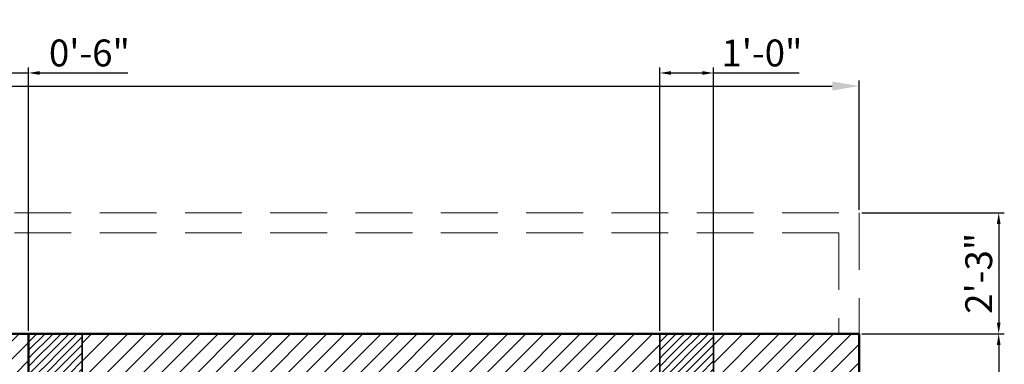
# Model space of a CAD drawing. Units: millimetres. Extents: x 225995 to 227247, y 225507 to 226008.
# Tile 10 of 23: x 226378 to 226598, y 225927 to 226004. Entities that reach past the tile are written whole.
import ezdxf

# ---------------------------------------------------------------- set-up
doc = ezdxf.new("R2010")
doc.units = ezdxf.units.MM
doc.linetypes.add('DASHED', pattern=[19.05, 12.7, -6.35])
for name, color, linetype, lineweight in [('A-ANNO-DIMS', 2, 'Continuous', 18), ('A-COLS', 40, 'Continuous', 35), ('A-WALL', 7, 'Continuous', 50), ('A-WALL-OVHD', 1, 'DASHED', 18), ('A-WALL-PATT', 8, 'Continuous', 13)]:
    doc.layers.add(name, color=color, linetype=linetype, lineweight=lineweight)
doc.styles.get("Standard").update_dxf_attribs({"font": 'arial.ttf'})
doc.dimstyles.new('ISO-25', dxfattribs={"dimtxt": 6, "dimasz": 2.5, "dimexe": 1.25, "dimexo": 0.625, "dimtad": 1, "dimdec": 0, "dimlunit": 3, "dimtxsty": 'Standard', "dimcen": 2.5, "dimadec": 0, "dimazin": 0, "dimtfac": 1, "dimtdec": 0, "dimtmove": 0, "dimatfit": 3, "dimfxl": 1, "dimarcsym": 0})
pattern_1 = [(45, (141, 234), (-0.898025612, 0.898025612), [])]
pattern_2 = [(45, (-6e-11, 234), (-0.898025612, 0.898025612), [])]

# ---------------------------------------------------------------- blocks, each defined once
blk = doc.blocks.new('*D68')
at = {"layer": 'A-ANNO-DIMS', "color": 0, "lineweight": -2, "transparency": 16777216}
for p, q in [((226033.88, 225961.4), (226033.88, 225990.31)), ((226565.88, 225961.4), (226565.88, 225990.31)), ((226039.88, 225989.06), (226559.88, 225989.06))]:
    blk.add_line(p, q, dxfattribs=at)
at = {"layer": 'A-ANNO-DIMS', "color": 0, "transparency": 16777216}
for points in [[(226039.88, 225990.06), (226039.88, 225988.06), (226033.88, 225989.06)], [(226559.88, 225990.06), (226559.88, 225988.06), (226565.88, 225989.06)]]:
    blk.add_solid(points, dxfattribs=at)
at = {"layer": 'Defpoints', "color": 0, "transparency": 16777216}
for p in [(226565.88, 225989.06), (226033.88, 225960.77), (226565.88, 225960.77)]:
    blk.add_point(p, dxfattribs=at)
at = {"layer": 'A-ANNO-DIMS', "color": 0, "transparency": 16777216, "insert": (226299.88, 225995.68), "char_height": 12, "attachment_point": 5}
blk.add_mtext('44\'-4"', dxfattribs=at)
blk = doc.blocks.new('*D96')
at = {"layer": 'A-ANNO-DIMS', "color": 0, "lineweight": -2, "transparency": 16777216}
for p, q in [((226371.88, 225991.97), (226369.38, 225991.97)), ((226374.38, 225934.4), (226374.38, 225993.22)), ((226374.38, 225991.97), (226380.38, 225991.97)), ((226380.38, 225934.4), (226380.38, 225993.22)), ((226382.88, 225991.97), (226402.58, 225991.97))]:
    blk.add_line(p, q, dxfattribs=at)
at = {"layer": 'A-ANNO-DIMS', "color": 0, "transparency": 16777216}
for points in [[(226371.88, 225992.39), (226371.88, 225991.56), (226374.38, 225991.97)], [(226382.88, 225992.39), (226382.88, 225991.56), (226380.38, 225991.97)]]:
    blk.add_solid(points, dxfattribs=at)
at = {"layer": 'Defpoints', "color": 0, "transparency": 16777216}
for p in [(226380.38, 225991.97), (226374.38, 225933.77), (226380.38, 225933.77)]:
    blk.add_point(p, dxfattribs=at)
at = {"layer": 'A-ANNO-DIMS', "color": 0, "transparency": 16777216, "insert": (226393.98, 225995.66), "char_height": 6, "attachment_point": 5}
blk.add_mtext('0\'-6"', dxfattribs=at)
blk = doc.blocks.new('*D97')
at = {"layer": 'A-ANNO-DIMS', "color": 0, "lineweight": -2, "transparency": 16777216}
for p, q in [((226521.38, 225934.4), (226521.38, 225993.22)), ((226523.88, 225991.97), (226530.88, 225991.97)), ((226533.38, 225934.4), (226533.38, 225993.22)), ((226533.38, 225991.97), (226552.51, 225991.97))]:
    blk.add_line(p, q, dxfattribs=at)
at = {"layer": 'A-ANNO-DIMS', "color": 0, "transparency": 16777216}
for points in [[(226523.88, 225992.39), (226523.88, 225991.56), (226521.38, 225991.97)], [(226530.88, 225992.39), (226530.88, 225991.56), (226533.38, 225991.97)]]:
    blk.add_solid(points, dxfattribs=at)
at = {"layer": 'Defpoints', "color": 0, "transparency": 16777216}
for p in [(226533.38, 225991.97), (226521.38, 225933.77), (226533.38, 225933.77)]:
    blk.add_point(p, dxfattribs=at)
at = {"layer": 'A-ANNO-DIMS', "color": 0, "transparency": 16777216, "insert": (226544.19, 225995.66), "char_height": 6, "attachment_point": 5}
blk.add_mtext('1\'-0"', dxfattribs=at)
blk = doc.blocks.new('*D98')
at = {"layer": 'A-ANNO-DIMS', "color": 0, "lineweight": -2, "transparency": 16777216}
for p, q in [((226566.5, 225960.77), (226598.33, 225960.77)), ((226597.08, 225958.27), (226597.08, 225936.27)), ((226566.5, 225933.77), (226598.33, 225933.77))]:
    blk.add_line(p, q, dxfattribs=at)
at = {"layer": 'A-ANNO-DIMS', "color": 0, "transparency": 16777216}
for points in [[(226596.66, 225958.27), (226597.49, 225958.27), (226597.08, 225960.77)], [(226596.66, 225936.27), (226597.49, 225936.27), (226597.08, 225933.77)]]:
    blk.add_solid(points, dxfattribs=at)
at = {"layer": 'Defpoints', "color": 0, "transparency": 16777216}
for p in [(226565.88, 225960.77), (226565.88, 225933.77), (226597.08, 225933.77)]:
    blk.add_point(p, dxfattribs=at)
at = {"layer": 'A-ANNO-DIMS', "color": 0, "transparency": 16777216, "insert": (226593.39, 225947.27), "char_height": 6, "attachment_point": 5, "rotation": 90}
blk.add_mtext('2\'-3"', dxfattribs=at)
blk = doc.blocks.new('*D99')
at = {"layer": 'A-ANNO-DIMS', "color": 0, "lineweight": -2, "transparency": 16777216}
for p, q in [((226566.5, 225933.77), (226598.33, 225933.77)), ((226597.08, 225931.27), (226597.08, 225879.27)), ((226566.5, 225876.77), (226598.33, 225876.77))]:
    blk.add_line(p, q, dxfattribs=at)
at = {"layer": 'A-ANNO-DIMS', "color": 0, "transparency": 16777216}
for points in [[(226596.66, 225931.27), (226597.49, 225931.27), (226597.08, 225933.77)], [(226596.66, 225879.27), (226597.49, 225879.27), (226597.08, 225876.77)]]:
    blk.add_solid(points, dxfattribs=at)
at = {"layer": 'Defpoints', "color": 0, "transparency": 16777216}
for p in [(226565.88, 225933.77), (226565.88, 225876.77), (226597.08, 225876.77)]:
    blk.add_point(p, dxfattribs=at)
at = {"layer": 'A-ANNO-DIMS', "color": 0, "transparency": 16777216, "insert": (226593.39, 225905.27), "char_height": 6, "attachment_point": 5, "rotation": 90}
blk.add_mtext('4\'-9"', dxfattribs=at)

msp = doc.modelspace()

# ---------------------------------------------------------------- hatches: boundary and pattern name
at = {"layer": 'A-WALL-PATT'}
h = msp.add_hatch(dxfattribs=at)
h.set_pattern_fill('ANSI31', color=256, scale=0.9)
h.paths.add_polyline_path([(226380.38, 225933.77), (226374.38, 225933.77), (226374.38, 225924.77), (226380.38, 225924.77)])
h = msp.add_hatch(dxfattribs=at)
h.set_pattern_fill('ANSI31', color=256, scale=0.4)
h.set_pattern_definition(pattern_2)
h.paths.add_polyline_path([(226384.88, 225933.77), (226380.38, 225933.77), (226380.38, 225929.27), (226384.88, 225929.27)])
h = msp.add_hatch(dxfattribs=at)
h.set_pattern_fill('ANSI31', color=256, scale=0.4)
h.set_pattern_definition(pattern_2)
h.paths.add_polyline_path([(226392.38, 225933.77), (226384.88, 225933.77), (226384.88, 225929.27), (226392.38, 225929.27)])
h = msp.add_hatch(dxfattribs=at)
h.set_pattern_fill('ANSI31', color=256, scale=0.9)
h.paths.add_polyline_path([(226521.38, 225933.77), (226392.38, 225933.77), (226392.38, 225924.77), (226521.38, 225924.77)])
h = msp.add_hatch(dxfattribs=at)
h.set_pattern_fill('ANSI31', color=256, scale=0.4)
h.set_pattern_definition(pattern_1)
h.paths.add_polyline_path([(226525.88, 225933.77), (226521.38, 225933.77), (226521.38, 225929.27), (226525.88, 225929.27)])
h = msp.add_hatch(dxfattribs=at)
h.set_pattern_fill('ANSI31', color=256, scale=0.4)
h.set_pattern_definition(pattern_1)
h.paths.add_polyline_path([(226533.38, 225933.77), (226525.88, 225933.77), (226525.88, 225929.27), (226533.38, 225929.27)])
h = msp.add_hatch(dxfattribs=at)
h.set_pattern_fill('ANSI31', color=256, scale=0.9)
h.paths.add_polyline_path([(226565.88, 225933.77), (226533.38, 225933.77), (226533.38, 225924.77), (226557.38, 225924.77), (226557.38, 225876.77), (226565.88, 225876.77)])
h = msp.add_hatch(dxfattribs=at)
h.set_pattern_fill('ANSI31', color=256, scale=0.4)
h.set_pattern_definition(pattern_2)
h.paths.add_polyline_path([(226384.88, 225929.27), (226380.38, 225929.27), (226380.38, 225924.77), (226384.88, 225924.77)])
h = msp.add_hatch(dxfattribs=at)
h.set_pattern_fill('ANSI31', color=256, scale=0.4)
h.set_pattern_definition(pattern_2)
h.paths.add_polyline_path([(226392.38, 225929.27), (226384.88, 225929.27), (226384.88, 225924.77), (226392.38, 225924.77)])
h = msp.add_hatch(dxfattribs=at)
h.set_pattern_fill('ANSI31', color=256, scale=0.4)
h.set_pattern_definition(pattern_1)
h.paths.add_polyline_path([(226525.88, 225929.27), (226521.38, 225929.27), (226521.38, 225924.77), (226525.88, 225924.77)])
h = msp.add_hatch(dxfattribs=at)
h.set_pattern_fill('ANSI31', color=256, scale=0.4)
h.set_pattern_definition(pattern_1)
h.paths.add_polyline_path([(226533.38, 225929.27), (226525.88, 225929.27), (226525.88, 225924.77), (226533.38, 225924.77)])

# ---------------------------------------------------------------- linework, layer by layer
at = {"layer": 'A-COLS'}
for points in [[(226380.38, 225924.77), (226380.38, 225933.77), (226392.38, 225933.77), (226392.38, 225924.77)], [(226521.38, 225924.77), (226521.38, 225933.77), (226533.38, 225933.77), (226533.38, 225924.77)]]:
    msp.add_lwpolyline(points, close=True, dxfattribs=at)
at = {"layer": 'A-WALL'}
for p, q in [((226565.88, 225933.77), (226236.38, 225933.77)), ((226243.88, 225933.77), (226565.88, 225933.77)), ((226380.38, 225933.77), (226380.38, 225924.77)), ((226565.88, 225933.77), (226565.88, 225570.77)), ((226565.88, 225570.77), (226565.88, 225933.77))]:
    msp.add_line(p, q, dxfattribs=at)
at = {"layer": 'A-WALL-OVHD'}
for p, q in [((226243.88, 225960.77), (226565.88, 225960.77)), ((226565.88, 225960.77), (226565.88, 225933.77)), ((226243.88, 225956.27), (226561.38, 225956.27)), ((226561.38, 225956.27), (226561.38, 225933.77))]:
    msp.add_line(p, q, dxfattribs=at)

# ---------------------------------------------------------------- dimensions: what is measured, and where the dimension line sits
at = {"layer": 'A-ANNO-DIMS'}
for base, p1, p2, override, picture, middle in [((226565.88, 225989.06), (226033.88, 225960.77), (226565.88, 225960.77), {"dimtxt": 12, "dimasz": 6, "dimclrd": 0, "dimclre": 0, "dimclrt": 0}, '*D68', (226299.88, 225995.68)), ((226380.38, 225991.97), (226374.38, 225933.77), (226380.38, 225933.77), {"dimdec": 1, "dimlfac": 1, "dimrnd": 0, "dimzin": 1, "dimdsep": 46, "dimlunit": 4, "dimfrac": 2}, '*D96', (226393.98, 225995.66)), ((226533.38, 225991.97), (226521.38, 225933.77), (226533.38, 225933.77), {"dimdec": 1, "dimlfac": 1, "dimrnd": 0, "dimzin": 1, "dimdsep": 46, "dimlunit": 4, "dimfrac": 2}, '*D97', (226544.19, 225995.66))]:
    dim = msp.add_linear_dim(base=base, p1=p1, p2=p2, dimstyle='ISO-25', override=override, dxfattribs=at)
    dim.commit()
    dim.dimension.update_dxf_attribs({"geometry": picture, "text_midpoint": middle})
for base, p1, p2, picture, middle in [((226597.08, 225933.77), (226565.88, 225960.77), (226565.88, 225933.77), '*D98', (226593.39, 225947.27)), ((226597.08, 225876.77), (226565.88, 225933.77), (226565.88, 225876.77), '*D99', (226593.39, 225905.27))]:
    dim = msp.add_linear_dim(base=base, p1=p1, p2=p2, angle=90, dimstyle='ISO-25', override={"dimdec": 1, "dimlfac": 1, "dimrnd": 0, "dimzin": 1, "dimdsep": 46, "dimlunit": 4, "dimfrac": 2}, dxfattribs=at)
    dim.commit()
    dim.dimension.update_dxf_attribs({"geometry": picture, "text_midpoint": middle})

doc.saveas('drawing.dxf')
